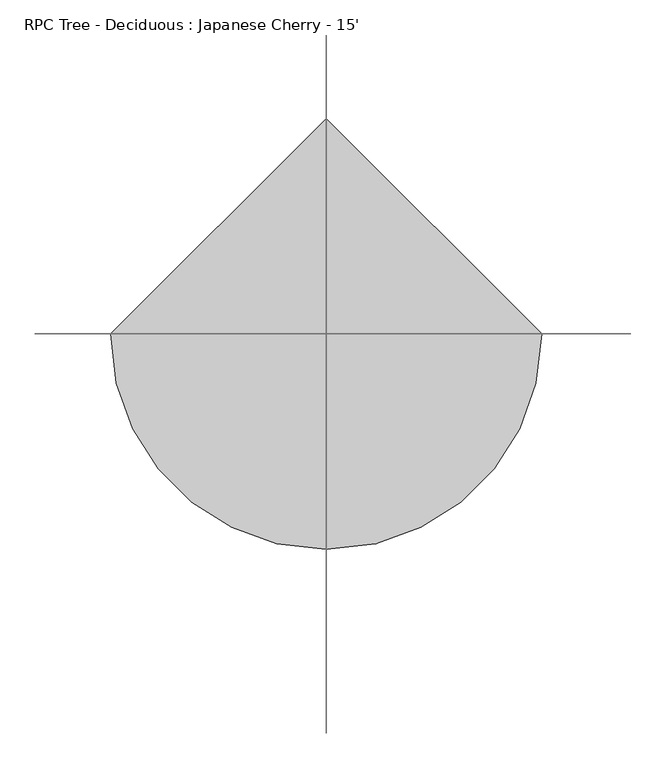
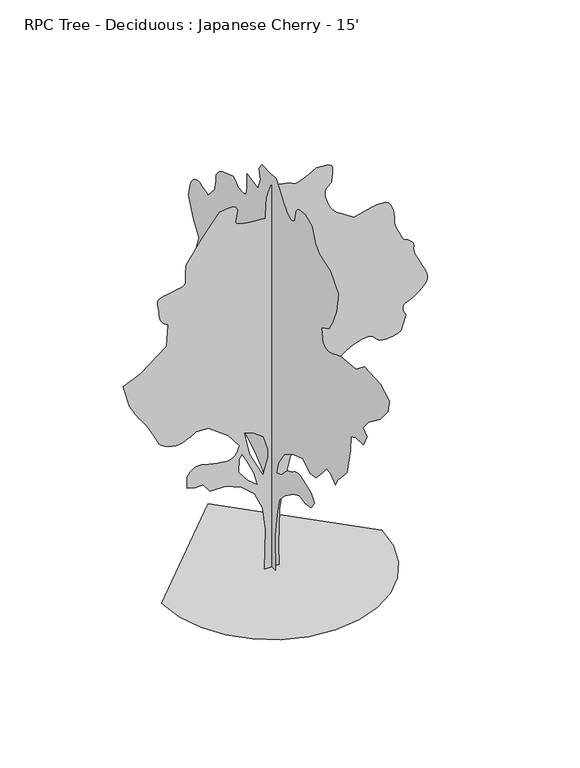
"""IFC4 building model written with IfcOpenShell, lengths in millimetres: geographic element geometry, RPC Tree - Deciduous : Japanese Cherry - 15'."""

from ifc_helpers import new_model, si_unit, origin, place, context, project, spatial, triangles, source, transform, mapped, element, save


def rpc_tree_deciduous_japanese_cherry_15_e499737d(model_context):
    return source(origin(), model_context, "Body", "Tessellation", [
        triangles([(-0.0028028, 75.7657196, 0.0059537), (-0.0028028, -73.2478183, 0.0059537), (-0.0028028, -59.7012251, 399.6312029), (-0.0028028, -100.3410047, 663.7914597), (-0.0028028, -147.7544623, 866.9916292), (-0.0028028, -256.1287339, 982.1375078), (-0.0028028, -418.6863261, 1097.2859299), (-0.0028028, -527.0605977, 1144.6976435), (-0.0028028, -635.434833, 1124.3775902), (-0.0028028, -750.5807842, 1144.6976435), (-0.0028028, -811.5407988, 1232.7519344), (-0.0028028, -750.5807842, 1314.0320023), (-0.0028028, -533.8347845, 1388.5377743), (-0.0028028, -514.9955638, 1387.0189716), (-0.0028028, -496.3341665, 1385.0834793), (-0.0028028, -478.0283798, 1382.3173691), (-0.0028028, -460.2559908, 1378.3091835), (-0.0028028, -443.1947865, 1372.6425236), (-0.0028028, -427.0200471, 1364.9005543), (-0.0028028, -411.9146828, 1354.6719635), (-0.0028028, -396.8067387, 1343.65345), (-0.0028028, -380.6345427, 1333.6991158), (-0.0028028, -363.5733384, 1324.6364422), (-0.0028028, -345.8009494, 1316.2824463), (-0.0028028, -327.4951627, 1308.4643188), (-0.0028028, -308.8337654, 1300.9992222), (-0.0028028, -289.994581, 1293.7118763), (-0.0028028, -188.3942419, 1185.3376774), (-0.0028028, -86.7944115, 1144.6976435), (-0.0028028, -127.4344454, 1286.9377258), (-0.0028028, -242.580869, 1456.2720119), (-0.0028028, -405.140496, 1557.8722057), (-0.0028028, -594.794799, 1618.8321476), (-0.0028028, -730.2607309, 1530.7779293), (-0.0028028, -838.6350025, 1544.3263756), (-0.0028028, -953.7809538, 1666.2439339), (-0.0028028, -1041.8351721, 1774.6181328), (-0.0028028, -1123.1126965, 1767.8439823), (-0.0028028, -1211.1669147, 1686.5663853), (-0.0028028, -1265.3528515, 1781.3922832), (-0.0028028, -1326.3127934, 1849.1240501), (-0.0028028, -1434.6871376, 1964.2723995), (-0.0028028, -1502.4187592, 2269.0726902), (-0.0028028, -1509.193055, 2431.6328259), (-0.0028028, -1604.0214237, 2472.2703163), (-0.0028028, -1753.0332584, 2485.8186172), (-0.0028028, -1813.9932003, 2614.5002975), (-0.0028028, -1739.4874283, 2675.4602394), (-0.0028028, -1841.0874767, 2797.3804138), (-0.0028028, -2071.3792339, 2973.5042564), (-0.0028028, -2220.3935394, 3149.6025192), (-0.0028028, -2247.4851997, 3291.8426743), (-0.0028028, -2078.1535297, 3386.6610146), (-0.0028028, -1766.5790886, 3400.2244308), (-0.0028028, -1610.7931034, 3278.3045471), (-0.0028028, -1312.7669632, 3244.4208595), (-0.0028028, -1272.2845505, 3228.5456657), (-0.0028028, -1232.7519344, 3213.2041603), (-0.0028028, -1195.1115721, 3198.9294502), (-0.0028028, -1160.3186377, 3186.2546425), (-0.0028028, -1129.3153702, 3175.7137161), (-0.0028028, -1103.0517843, 3167.8397781), (-0.0028028, -1082.4726625, 3163.1406464), (-0.0028028, -1064.0500225, 3162.8865921), (-0.0028028, -1044.5580437, 3166.9000099), (-0.0028028, -1025.4242552, 3173.6309944), (-0.0028028, -1008.065867, 3181.5558014), (-0.0028028, -993.907865, 3189.1248161), (-0.0028028, -984.3701477, 3194.789296), (-0.0028028, -980.8726141, 3197.024334), (-0.0028028, -947.0067307, 3359.5844696), (-0.0028028, -1089.2468857, 3434.0828293), (-0.0028028, -1156.9810507, 3542.4645859), (-0.0028028, -1231.4868954, 3718.5628487), (-0.0028028, -1272.127002, 3942.0832169), (-0.0028028, -1116.3410168, 4118.1814796), (-0.0028028, -913.1409199, 4192.7051285), (-0.0028028, -831.8608521, 4267.2034882), (-0.0028028, -770.9007648, 4429.7636238), (-0.0028028, -628.6606825, 4483.9417122), (-0.0028028, -605.4958537, 4483.8402649), (-0.0028028, -582.6891789, 4483.1542603), (-0.0028028, -560.5911455, 4481.2747238), (-0.0028028, -539.5599438, 4477.6426781), (-0.0028028, -519.9511116, 4471.5974075), (-0.0028028, -502.1202959, 4462.6310944), (-0.0028028, -486.4205638, 4450.0836044), (-0.0028028, -473.6824242, 4434.3863068), (-0.0028028, -464.1447433, 4416.5554184), (-0.0028028, -457.2740144, 4396.9467316), (-0.0028028, -452.5343691, 4375.9154572), (-0.0028028, -449.3949532, 4353.8173874), (-0.0028028, -447.3197528, 4331.0083145), (-0.0028028, -445.7805299, 4307.8434494), (-0.0028028, -434.0914178, 4294.9401672), (-0.0028028, -421.9248276, 4283.0531021), (-0.0028028, -408.8133096, 4273.1978897), (-0.0028028, -394.279422, 4266.3398781), (-0.0028028, -377.850701, 4263.5202827), (-0.0028028, -359.0495956, 4265.7303223), (-0.0028028, -337.4062583, 4273.9853416), (-0.0028028, -315.9610193, 4285.9741447), (-0.0028028, -297.7161846, 4298.6995308), (-0.0028028, -282.1358129, 4312.0091835), (-0.0028028, -268.6864885, 4325.8013649), (-0.0028028, -256.8373934, 4339.9237587), (-0.0028028, -246.0563473, 4354.3002068), (-0.0028028, -235.8074452, 4368.8033913), (-0.0028028, -140.9810386, 4497.5054192), (-0.0028028, -80.0209877, 4572.0037788), (-0.0028028, 21.579147, 4565.2219254), (-0.0028028, 184.1389784, 4572.0037788), (-0.0028028, 245.0987749, 4490.7235657), (-0.0028028, 218.0055885, 4375.5852448), (-0.0028028, 265.4200454, 4246.8835075), (-0.0028028, 475.3918765, 4287.5234688), (-0.0028028, 475.3918765, 4138.5014603), (-0.0028028, 476.9514107, 4115.4383331), (-0.0028028, 479.1637756, 4093.1623672), (-0.0028028, 482.6791134, 4072.5630432), (-0.0028028, 488.1502911, 4054.4781006), (-0.0028028, 496.2249435, 4039.6699928), (-0.0028028, 507.5609885, 4029.0273285), (-0.0028028, 522.8060609, 4023.3631393), (-0.0028028, 540.2228757, 4021.2551285), (-0.0028028, 557.6396542, 4020.5691238), (-0.0028028, 575.056469, 4021.0519432), (-0.0028028, 592.4732474, 4022.4995293), (-0.0028028, 609.8900259, 4024.6586998), (-0.0028028, 627.3093842, 4027.2748192), (-0.0028028, 644.726199, 4030.1449928), (-0.0028028, 660.7002239, 4045.9437378), (-0.0028028, 676.7352917, 4060.8791634), (-0.0028028, 692.8896835, 4074.0362091), (-0.0028028, 709.2193554, 4084.5265572), (-0.0028028, 725.7878208, 4091.4607269), (-0.0028028, 742.6534338, 4093.9498192), (-0.0028028, 759.8720776, 4091.1049347), (-0.0028028, 942.7522665, 4030.1449928), (-0.0028028, 968.7009007, 4012.6698967), (-0.0028028, 993.5827394, 3994.8390083), (-0.0028028, 1016.3309875, 3976.2971169), (-0.0028028, 1035.8813931, 3956.6881393), (-0.0028028, 1051.1646172, 3935.6568649), (-0.0028028, 1061.1163353, 3912.8477921), (-0.0028028, 1064.6722956, 3887.9048378), (-0.0028028, 1065.462291, 3862.3526184), (-0.0028028, 1067.6745832, 3837.8921928), (-0.0028028, 1071.0705969, 3814.3209572), (-0.0028028, 1075.4140091, 3791.4610153), (-0.0028028, 1080.4685698, 3769.1088913), (-0.0028028, 1085.9981741, 3747.1381393), (-0.0028028, 1091.7640285, 3725.3447021), (-0.0028028, 1220.4582081, 3583.1045471), (-0.0028028, 1259.5970982, 3600.2497215), (-0.0028028, 1298.4413841, 3615.8705704), (-0.0028028, 1336.691375, 3628.418351), (-0.0028028, 1374.0521759, 3636.343158), (-0.0028028, 1410.2294735, 3638.0956673), (-0.0028028, 1444.9259022, 3632.1521347), (-0.0028028, 1477.8442417, 3616.9629456), (-0.0028028, 1506.4193871, 3593.4931572), (-0.0028028, 1528.9517326, 3564.3086014), (-0.0028028, 1546.4471764, 3530.3996246), (-0.0028028, 1559.9143776, 3492.7059952), (-0.0028028, 1570.361269, 3452.1674812), (-0.0028028, 1578.7941845, 3409.7241417), (-0.0028028, 1586.218586, 3366.3410339), (-0.0028028, 1498.1643677, 3136.0643921), (-0.0028028, 1389.7926395, 2987.0423836), (-0.0028028, 1477.8442417, 2743.2023254), (-0.0028028, 1396.5641739, 2614.5002975), (-0.0028028, 1363.3893093, 2602.8164177), (-0.0028028, 1331.4588455, 2590.6497185), (-0.0028028, 1302.0151485, 2577.543251), (-0.0028028, 1276.3027645, 2563.0144867), (-0.0028028, 1255.5687103, 2546.5806061), (-0.0028028, 1241.0552067, 2527.7820442), (-0.0028028, 1234.0040382, 2506.1385979), (-0.0028028, 1231.6953129, 2483.1135498), (-0.0028028, 1230.4506214, 2460.4416779), (-0.0028028, 1230.0949745, 2438.0692062), (-0.0028028, 1230.4506214, 2415.9330574), (-0.0028028, 1231.339666, 2393.9721886), (-0.0028028, 1232.5842121, 2372.13326), (-0.0028028, 1234.0040382, 2350.3502872), (-0.0028028, 1206.9124506, 2241.9785591), (-0.0028028, 1017.2581112, 2262.2985397), (-0.0028028, 1001.4999161, 2230.5052769), (-0.0028028, 986.9863398, 2199.5401611), (-0.0028028, 974.9594576, 2170.2361359), (-0.0028028, 966.6663591, 2143.4188774), (-0.0028028, 963.3491198, 2119.9211838), (-0.0028028, 966.2523582, 2100.5664059), (-0.0028028, 976.6180773, 2086.1925739), (-0.0028028, 993.4227201, 2074.2646683), (-0.0028028, 1014.0196461, 2062.1005852), (-0.0028028, 1037.2225176, 2050.292149), (-0.0028028, 1061.8478313, 2039.431184), (-0.0028028, 1086.7093952, 2030.1093693), (-0.0028028, 1110.6234879, 2022.9211452), (-0.0028028, 1132.4039898, 2018.4583363), (-0.0028028, 1152.1322187, 2014.567004), (-0.0028028, 1170.7936523, 2008.9003441), (-0.0028028, 1188.5660414, 2001.7526699), (-0.0028028, 1205.6272093, 1993.4190216), (-0.0028028, 1222.157523, 1984.1961834), (-0.0028028, 1238.3297916, 1974.3816662), (-0.0028028, 1254.3241642, 1964.2723995), (-0.0028028, 1410.1126202, 2045.5524673), (-0.0028028, 1454.8979679, 2056.9850544), (-0.0028028, 1498.4412403, 2067.3533169), (-0.0028028, 1539.4952751, 2075.5879887), (-0.0028028, 1576.817997, 2080.6222744), (-0.0028028, 1609.1650051, 2081.3919949), (-0.0028028, 1635.2914627, 2076.8326801), (-0.0028028, 1653.9502075, 2065.8725933), (-0.0028028, 1666.2946575, 2049.9747265), (-0.0028028, 1674.7249569, 2031.5900928), (-0.0028028, 1679.8989143, 2011.1329113), (-0.0028028, 1682.4669262, 1989.0146393), (-0.0028028, 1683.0789528, 1965.6542919), (-0.0028028, 1682.3881519, 1941.4631813), (-0.0028028, 1681.0444839, 1916.8582878), (-0.0028028, 1657.7627655, 1892.3904499), (-0.0028028, 1634.1255455, 1869.1697742), (-0.0028028, 1609.7770317, 1848.4331039), (-0.0028028, 1584.3618679, 1831.4303627), (-0.0028028, 1557.5241165, 1819.4059513), (-0.0028028, 1528.9110374, 1813.5996197), (-0.0028028, 1498.1643677, 1815.2582394), (-0.0028028, 1465.6015297, 1822.4057682), (-0.0028028, 1432.5637207, 1830.9782101), (-0.0028028, 1400.2370602, 1839.0732101), (-0.0028028, 1369.8078129, 1844.8009129), (-0.0028028, 1342.4571568, 1846.2614342), (-0.0028028, 1319.3735367, 1841.5624477), (-0.0028028, 1301.7382759, 1828.8040695), (-0.0028028, 1288.4084209, 1812.3752758), (-0.0028028, 1277.2120113, 1797.7219551), (-0.0028028, 1267.7912201, 1784.5521194), (-0.0028028, 1259.7953419, 1772.5657871), (-0.0028028, 1252.8636429, 1761.4660286), (-0.0028028, 1246.6430923, 1750.9605652), (-0.0028028, 1240.778334, 1740.752322), (-0.0028028, 1263.8618088, 1737.6916077), (-0.0028028, 1286.1172817, 1733.6834221), (-0.0028028, 1306.714135, 1727.7779686), (-0.0028028, 1324.821896, 1719.0302467), (-0.0028028, 1339.6122723, 1706.4901691), (-0.0028028, 1350.2574074, 1689.2105553), (-0.0028028, 1355.9242126, 1666.2439339), (-0.0028028, 1358.2355541, 1639.3300243), (-0.0028028, 1359.4802456, 1610.9912018), (-0.0028028, 1359.8357471, 1581.4687305), (-0.0028028, 1359.4802456, 1550.9989334), (-0.0028028, 1358.591201, 1519.8178425), (-0.0028028, 1357.3466549, 1488.1643967), (-0.0028028, 1355.9242126, 1456.2720119), (-0.0028028, 1321.1312782, 1430.3436527), (-0.0028028, 1286.5720505, 1405.5990875), (-0.0028028, 1252.4876484, 1383.2266159), (-0.0028028, 1219.1146128, 1364.4078518), (-0.0028028, 1186.6915192, 1350.328624), (-0.0028028, 1155.4494581, 1342.1725811), (-0.0028028, 1125.6323828, 1341.1261333), (-0.0028028, 1095.812764, 1344.8167511), (-0.0028028, 1064.5732464, 1349.9322819), (-0.0028028, 1032.1476093, 1356.2316067), (-0.0028028, 998.774501, 1363.478112), (-0.0028028, 964.6902443, 1371.4385273), (-0.0028028, 930.1334873, 1379.8688267), (-0.0028028, 895.3380095, 1388.5377743), (-0.0028028, 692.1378399, 1341.1261333), (-0.0028028, 455.0718596, 1219.2061043), (-0.0028028, 319.6059277, 1144.6976435), (-0.0028028, 163.8189614, 1016.005862), (-0.0028028, 68.9922959, 819.5799156), (-0.0028028, 41.8991095, 541.8713216), (-0.0028028, 68.9922959, 264.1652892), (80.2102203, 0.0002552, 0.0), (-82.349661, 0.0002552, 0.0), (-68.8030678, 0.0002233, 460.5862032), (-102.6694236, 0.000202, 724.7463873), (-190.7229152, 0.0001914, 914.3981833), (-332.9637969, 0.0001914, 1043.0925081), (-509.0697627, 0.0001807, 1117.5983528), (-678.4015417, 0.0001807, 1117.5983528), (-759.684153, 0.0001807, 1219.1984013), (-847.7358278, 0.0001807, 1219.1984013), (-935.7901188, 0.0001807, 1239.5183819), (-935.7901188, 0.0001701, 1368.2127068), (-918.2539072, 0.0001701, 1391.2175526), (-900.0065472, 0.0001701, 1412.9192802), (-880.3392883, 0.0001595, 1432.0150623), (-858.5384388, 0.0001595, 1447.2017807), (-833.8928501, 0.0001595, 1457.1737011), (-805.6936993, 0.0001595, 1460.6307575), (-773.2299831, 0.0001595, 1456.266925), (-734.6829174, 0.0001595, 1446.5108345), (-690.4487715, 0.0001595, 1435.4516258), (-643.1335636, 0.0001701, 1424.2757092), (-595.3460009, 0.0001701, 1414.1639717), (-549.689449, 0.0001701, 1406.3051491), (-508.7725788, 0.0001701, 1401.8804192), (-475.2013721, 0.0001701, 1402.0785175), (-448.544024, 0.0001701, 1408.1415195), (-426.1513865, 0.0001701, 1419.8916744), (-407.3122021, 0.0001595, 1436.3813656), (-391.3152497, 0.0001595, 1456.660651), (-377.4544679, 0.0001595, 1479.7848209), (-365.0135485, 0.0001595, 1504.8039333), (-353.2838139, 0.0001595, 1530.7728424), (-475.2013721, 0.0001488, 1693.3329781), (-698.7215223, 0.0001382, 1855.8931137), (-834.1899977, 0.0001382, 1862.6647934), (-856.0492739, 0.0001382, 1849.6320133), (-878.4419477, 0.0001382, 1836.7771294), (-901.9038877, 0.0001382, 1824.277747), (-926.9610065, 0.0001382, 1812.3092915), (-954.1543322, 0.0001382, 1801.0544552), (-984.01203, 0.0001382, 1790.6861927), (-1017.0701866, 0.0001488, 1781.3847256), (-1055.1015862, 0.0001488, 1778.1664627), (-1097.4002398, 0.0001488, 1784.6638859), (-1140.7656887, 0.0001382, 1798.9792912), (-1182.0000904, 0.0001382, 1819.2206429), (-1217.9005154, 0.0001382, 1843.490237), (-1245.2690483, 0.0001382, 1869.8935673), (-1260.907774, 0.0001382, 1896.5332203), (-1274.5551968, 0.0001382, 1929.7461639), (-1296.2570698, 0.0001276, 1973.9803825), (-1323.2903034, 0.0001276, 2024.4959038), (-1352.9320988, 0.0001276, 2076.5482498), (-1382.45457, 0.0001276, 2125.4025352), (-1409.1321568, 0.0001169, 2166.3195145), (-1430.2420601, 0.0001169, 2194.5592152), (-1448.055217, 0.0001169, 2217.0508656), (-1466.5769062, 0.0001169, 2243.4541958), (-1485.6928905, 0.0001169, 2273.113868), (-1505.2813751, 0.0001169, 2305.3794857), (-1525.2255066, 0.0001063, 2339.6035595), (-1545.4082863, 0.0001063, 2375.12799), (-1565.7080647, 0.0001063, 2411.3051422), (-1640.2164528, 9.57e-05, 2668.7039658), (-1443.7878902, 8.51e-05, 2749.9838882), (-1159.310269, 7.44e-05, 2973.5042564), (-1145.7618954, 5.32e-05, 3217.3190254), (-1165.9447477, 5.32e-05, 3231.9748169), (-1185.2970549, 5.32e-05, 3247.3163223), (-1202.9906696, 5.32e-05, 3264.0804153), (-1218.1951195, 5.32e-05, 3282.9780991), (-1230.0823299, 5.32e-05, 3304.7203766), (-1237.8242992, 5.32e-05, 3330.0188324), (-1240.5902641, 5.32e-05, 3359.5591805), (-1243.0389519, 4.25e-05, 3392.8330215), (-1248.5659401, 4.25e-05, 3427.5294502), (-1254.4511913, 4.25e-05, 3461.7686394), (-1257.9665291, 4.25e-05, 3493.6204742), (-1256.3865383, 4.25e-05, 3521.204837), (-1246.9860947, 4.25e-05, 3542.6169022), (-1227.0419632, 4.25e-05, 3556.002713), (-1192.1092844, 4.25e-05, 3564.4103394), (-1144.1438982, 3.19e-05, 3572.715937), (-1090.0164608, 3.19e-05, 3581.5808029), (-1036.6002445, 3.19e-05, 3591.7915169), (-990.7659056, 3.19e-05, 3603.9835052), (-959.3867163, 3.19e-05, 3618.9186401), (-949.3359489, 3.19e-05, 3637.2829262), (-951.449192, 3.19e-05, 3659.3809959), (-952.1400656, 3.19e-05, 3684.6794518), (-951.644747, 3.19e-05, 3712.6448959), (-950.2045732, 3.19e-05, 3742.718351), (-948.0532511, 2.13e-05, 3774.4175789), (-945.4268852, 2.13e-05, 3807.1836021), (-942.5617258, 2.13e-05, 3840.4830231), (-773.2299831, 1.06e-05, 4084.3233719), (-576.803964, -1.06e-05, 4328.16343), (-534.9980856, -1.06e-05, 4335.1231796), (-494.9117606, -1.06e-05, 4340.3809982), (-458.2595647, -1.06e-05, 4342.2096657), (-426.7635221, -1.06e-05, 4338.8569633), (-402.1382083, -1.06e-05, 4328.6459587), (-386.1031769, -1.06e-05, 4309.850013), (-380.3754742, 0.0, 4280.7416153), (-383.1999384, 0.0, 4247.9503029), (-389.6972889, 0.0, 4219.0450905), (-396.9057878, 0.0, 4193.848082), (-401.8613357, 0.0, 4172.0549355), (-401.6048106, 0.0, 4153.462175), (-393.1720041, 0.0, 4137.8410355), (-373.6038308, 0.0, 4124.9633331), (-343.9238837, 0.0, 4114.5238541), (-307.8431645, 0.0, 4106.2435455), (-266.4335192, 1.06e-05, 4099.7157463), (-220.7586908, 1.06e-05, 4094.6355331), (-171.883967, 1.06e-05, 4090.5971169), (-120.8766607, 1.06e-05, 4087.2697037), (-68.8030678, 1.06e-05, 4084.3233719), (-62.0293897, 0.0, 4267.2034882), (-60.4495079, -1.06e-05, 4293.1367889), (-56.0260951, -1.06e-05, 4318.689299), (-49.2331141, -1.06e-05, 4343.962175), (-40.544273, -1.06e-05, 4369.0065765), (-30.4335416, -1.06e-05, 4393.8733727), (-19.3751868, -1.06e-05, 4418.612851), (-7.8427643, -1.06e-05, 4443.3017509), (38.3857792, -1.06e-05, 4434.5642029), (83.3110485, -1.06e-05, 4425.7249168), (125.6295138, -1.06e-05, 4416.6571564), (164.0381523, -1.06e-05, 4407.2083145), (197.2334371, -1.06e-05, 4397.3022331), (223.9120957, -1.06e-05, 4386.7865959), (242.7705922, -1.06e-05, 4375.5599556), (267.3174405, -1.06e-05, 4372.2834114), (307.2640574, -1.06e-05, 4382.5194145), (355.6256767, -1.06e-05, 4401.5188362), (405.4097383, -1.06e-05, 4424.5566742), (449.6235366, -1.06e-05, 4446.8576385), (481.2770551, -2.13e-05, 4463.7234695), (493.3827115, -2.13e-05, 4470.4035851), (503.1388384, -2.13e-05, 4470.6067703), (528.2975498, -2.13e-05, 4470.3274269), (562.6967946, -2.13e-05, 4468.2699944), (600.177065, -2.13e-05, 4463.1392029), (634.5763098, -1.06e-05, 4453.6142029), (659.7350212, -1.06e-05, 4438.3994339), (669.4911844, -1.06e-05, 4416.1999168), (669.0949877, -1.06e-05, 4390.4698013), (667.9900406, -1.06e-05, 4365.4506889), (666.2907984, -1.06e-05, 4341.0411324), (664.1190559, -1.06e-05, 4317.089106), (661.5918119, -1.06e-05, 4293.4922905), (658.8257017, 0.0, 4270.1245308), (655.9428108, 0.0, 4246.8835075), (638.6835445, 0.0, 4233.6753021), (622.3741476, 0.0, 4219.7308044), (607.9571134, 0.0, 4204.2114029), (596.3848546, 0.0, 4186.4060944), (588.6048426, 0.0, 4165.5271362), (585.5644395, 0.0, 4140.7876579), (588.2111166, 0.0, 4111.3996262), (595.5949319, 1.06e-05, 4078.8367882), (605.8235227, 1.06e-05, 4045.6643944), (618.4244614, 1.06e-05, 4012.9492401), (632.9176901, 1.06e-05, 3981.7834099), (648.8333611, 1.06e-05, 3953.233699), (665.698974, 1.06e-05, 3928.3416138), (683.0370146, 2.13e-05, 3908.1995293), (703.4154945, 2.13e-05, 3889.8099541), (729.1278786, 2.13e-05, 3869.6170006), (759.2802532, 2.13e-05, 3847.9505905), (792.9912043, 2.13e-05, 3825.1159378), (829.3639841, 2.13e-05, 3801.3670967), (867.5148531, 2.13e-05, 3777.0592781), (906.5572374, 2.13e-05, 3752.4212471), (974.48703, 2.13e-05, 3771.0140076), (1040.6997763, 2.13e-05, 3787.8795479), (1103.475959, 2.13e-05, 3801.2909386), (1161.1010027, 2.13e-05, 3809.5712471), (1211.8502306, 2.13e-05, 3810.9682549), (1254.0116833, 2.13e-05, 3803.7800308), (1285.8633728, 2.13e-05, 3786.2793549), (1308.8096466, 2.13e-05, 3757.831382), (1325.9495888, 3.19e-05, 3721.2045479), (1338.1136719, 3.19e-05, 3679.8280037), (1346.1325138, 3.19e-05, 3637.155899), (1350.8315002, 3.19e-05, 3596.6173851), (1353.0438652, 4.25e-05, 3561.641613), (1353.5976105, 4.25e-05, 3535.6827324), (1358.8503422, 4.25e-05, 3507.9969223), (1372.3961723, 4.25e-05, 3469.2870758), (1390.9178616, 4.25e-05, 3425.1418053), (1411.1006413, 5.32e-05, 3381.0982727), (1429.6249466, 5.32e-05, 3342.7442184), (1443.1707767, 5.32e-05, 3315.6423843), (1448.4235085, 5.32e-05, 3305.3808014), (1455.5126106, 5.32e-05, 3302.5614967), (1473.6202263, 5.32e-05, 3294.4079247), (1498.0094353, 5.32e-05, 3281.4031952), (1523.9376492, 5.32e-05, 3264.0042572), (1546.6656223, 5.32e-05, 3242.6936394), (1561.456144, 5.32e-05, 3217.9538704), (1563.5693871, 6.38e-05, 3190.2424805), (1560.9227463, 6.38e-05, 3161.8962456), (1563.9655838, 6.38e-05, 3134.3880409), (1571.7456322, 6.38e-05, 3106.8795456), (1583.3178909, 6.38e-05, 3078.5585999), (1597.7324181, 6.38e-05, 3048.5613029), (1614.0443584, 7.44e-05, 3016.0746231), (1631.3036247, 7.44e-05, 2980.2605301), (1651.0114334, 7.44e-05, 2941.4239471), (1672.8529781, 7.44e-05, 2900.911013), (1693.1526112, 7.44e-05, 2859.5850471), (1708.2377369, 8.51e-05, 2818.2593719), (1714.4404106, 8.51e-05, 2777.7461472), (1708.0801884, 8.51e-05, 2738.9095642), (1685.4894161, 8.51e-05, 2702.5620735), (1655.0603142, 9.57e-05, 2670.8884254), (1626.9983643, 9.57e-05, 2644.9042557), (1600.3587112, 9.57e-05, 2623.6442162), (1574.1941746, 9.57e-05, 2606.1944092), (1547.5546669, 9.57e-05, 2591.5894867), (1519.4951878, 9.57e-05, 2578.8641006), (1489.0634697, 9.57e-05, 2567.103772), (1463.2545799, 9.57e-05, 2553.5147758), (1448.4615875, 9.57e-05, 2536.3646599), (1442.8532089, 9.57e-05, 2516.2632706), (1444.5930737, 0.0001063, 2493.7893517), (1451.8397243, 0.0001063, 2469.5399597), (1462.7592613, 0.0001063, 2444.1069191), (1475.5176395, 0.0001063, 2418.079438), (1421.329232, 0.0001169, 2248.7450066), (1402.2741451, 0.0001169, 2240.1167542), (1382.0913654, 0.0001169, 2231.9607113), (1359.6579964, 0.0001169, 2224.752285), (1333.8491066, 0.0001169, 2218.9661556), (1303.5367126, 0.0001169, 2215.0772942), (1267.5955925, 0.0001169, 2213.5558754), (1224.9032856, 0.0001169, 2214.8791958), (1186.5543182, 0.0001169, 2223.6651421), (1160.2907324, 0.0001169, 2241.2216286), (1139.9504042, 0.0001169, 2263.0426804), (1119.3738258, 0.0001169, 2284.6250839), (1092.3990189, 0.0001169, 2301.470422), (1052.8638594, 0.0001169, 2309.0727196), (994.6089123, 0.0001169, 2302.9309433), (927.2531399, 0.0001169, 2283.7970821), (865.4625074, 0.0001169, 2256.8426228), (810.6645441, 0.0001169, 2224.1985397), (764.2764599, 0.0001169, 2188.0035107), (727.7258566, 0.0001169, 2150.3835686), (702.4274008, 0.0001276, 2113.4772457), (689.8112377, 0.0001276, 2079.4133366), (689.5343651, 0.0001276, 2049.0602474), (699.2092106, 0.0001276, 2021.5520428), (717.179698, 0.0001276, 1996.4136063), (741.7847368, 0.0001276, 1973.172583), (771.3655621, 0.0001382, 1951.3515312), (804.2662428, 0.0001382, 1930.4778053), (838.8229998, 0.0001382, 1910.0790504), (858.9855045, 0.0001382, 1896.9268009), (878.2006107, 0.0001382, 1883.2412991), (895.5183764, 0.0001382, 1868.4914726), (909.9938009, 0.0001382, 1852.1415985), (920.6770878, 0.0001382, 1833.6579884), (926.620693, 0.0001382, 1812.5073898), (926.8772181, 0.0001382, 1788.158876), (924.1721506, 0.0001488, 1758.4790016), (921.8225847, 0.0001488, 1722.4008259), (919.7677683, 0.0001488, 1680.9911442), (917.9516727, 0.0001488, 1635.3142811), (916.3107845, 0.0001595, 1586.4395027), (914.7919092, 0.0001595, 1535.4337498), (913.3288445, 0.0001595, 1483.3585854), (878.4571358, 0.0001595, 1457.529348), (843.3467062, 0.0001595, 1433.4780544), (807.7613056, 0.0001701, 1412.980323), (771.4646839, 0.0001701, 1397.8139523), (734.2231344, 0.0001701, 1389.7570312), (695.792922, 0.0001701, 1390.585033), (655.9428108, 0.0001701, 1402.0785175), (615.8971447, 0.0001701, 1417.3236626), (576.9157305, 0.0001701, 1428.6597439), (538.820781, 0.0001595, 1436.7368671), (501.4395962, 0.0001595, 1442.205574), (464.5917727, 0.0001595, 1445.7209118), (428.0995597, 0.0001595, 1447.9332767), (391.7826267, 0.0001595, 1449.4927746), (276.6366936, 0.0001701, 1374.9868572), (202.1305764, 0.0001807, 1205.6525711), (127.6236689, 0.0001914, 921.1724064), (86.9838894, 0.0002126, 643.4663195), (73.4370464, 0.0002339, 237.0665254), (-95.8962542, 8.51e-05, 1097.2783722), (-41.7096271, 7.44e-05, 1286.9326389), (-41.7096271, 6.38e-05, 1381.7585369), (-89.122576, 5.32e-05, 1544.3186726), (-211.0424234, 5.32e-05, 1632.3728909), (-305.8695931, 5.32e-05, 1666.238847), (-244.9095423, 6.38e-05, 1395.3069832), (-156.8557963, 6.38e-05, 1009.2266247), (-197.4958302, 6.38e-05, 1158.2383867), (-272.003746, 5.32e-05, 1320.7984497), (-326.1896101, 4.25e-05, 1422.3986435), (-360.0554572, 4.25e-05, 1374.9868572), (-366.829644, 5.32e-05, 1225.9725517), (-265.2295592, 6.38e-05, 1097.2783722), (-1212.9170259, 0.0, 0.0045929), (-1180.85205, -277.9194097, 0.0045929), (-1089.5287725, -533.1464181, 0.0045929), (-946.2625174, -758.3633034, 0.0045929), (-758.3633034, -946.2625174, 0.0045929), (-533.1464181, -1089.5287725, 0.0045929), (-277.9194097, -1180.85205, 0.0045929), (5.3e-05, -1212.9170259, 0.0045929), (277.9194097, -1180.85205, 0.0045929), (533.1464181, -1089.5287725, 0.0045929), (758.3633034, -946.2625174, 0.0045929), (946.2625174, -758.3633034, 0.0045929), (1089.5287725, -533.1464181, 0.0045929), (1180.85205, -277.9194097, 0.0045929), (1212.9170259, 0.0001063, 0.0045929), (-0.0001591, 1212.9170259, 0.0045929)], [[38, 39, 40], [115, 116, 117], [1, 2, 3], [280, 1, 3], [279, 280, 3], [279, 3, 4], [278, 279, 4], [278, 4, 5], [186, 187, 188], [277, 278, 5], [46, 47, 48], [45, 46, 48], [277, 5, 6], [185, 186, 188], [10, 11, 12], [9, 10, 12], [9, 12, 13], [8, 9, 13], [8, 13, 14], [8, 14, 15], [8, 15, 16], [8, 16, 17], [8, 17, 18], [8, 18, 19], [8, 19, 20], [8, 20, 21], [7, 8, 21], [7, 21, 22], [7, 22, 23], [7, 23, 24], [7, 24, 25], [7, 25, 26], [6, 7, 26], [6, 26, 27], [6, 27, 28], [277, 6, 28], [277, 28, 29], [51, 52, 53], [50, 51, 53], [50, 53, 54], [50, 54, 55], [49, 50, 55], [49, 55, 56], [48, 49, 56], [48, 56, 57], [45, 48, 57], [44, 45, 57], [44, 57, 58], [44, 58, 59], [44, 59, 60], [44, 60, 61], [44, 61, 62], [44, 62, 63], [276, 277, 29], [276, 29, 30], [184, 185, 188], [183, 184, 188], [44, 63, 64], [115, 117, 118], [111, 112, 113], [111, 113, 114], [182, 183, 188], [109, 110, 111], [109, 111, 114], [108, 109, 114], [108, 114, 115], [107, 108, 115], [106, 107, 115], [105, 106, 115], [104, 105, 115], [115, 118, 119], [170, 171, 172], [170, 172, 173], [170, 173, 174], [170, 174, 175], [74, 75, 76], [74, 76, 77], [73, 74, 77], [72, 73, 77], [71, 72, 77], [258, 259, 260], [181, 182, 188], [78, 79, 80], [170, 175, 176], [103, 104, 115], [78, 80, 81], [44, 64, 65], [275, 276, 30], [275, 30, 31], [274, 275, 31], [78, 81, 82], [78, 82, 83], [78, 83, 84], [78, 84, 85], [78, 85, 86], [78, 86, 87], [78, 87, 88], [78, 88, 89], [78, 89, 90], [78, 90, 91], [78, 91, 92], [78, 92, 93], [78, 93, 94], [78, 94, 95], [78, 95, 96], [71, 77, 78], [71, 78, 96], [71, 96, 97], [71, 97, 98], [71, 98, 99], [71, 99, 100], [115, 119, 120], [180, 181, 188], [38, 40, 41], [223, 224, 225], [33, 34, 35], [33, 35, 36], [33, 36, 37], [102, 103, 115], [179, 180, 188], [44, 65, 66], [170, 176, 177], [71, 100, 101], [43, 44, 66], [42, 43, 66], [41, 42, 66], [38, 41, 66], [37, 38, 66], [33, 37, 66], [33, 66, 67], [33, 67, 68], [33, 68, 69], [33, 69, 70], [32, 33, 70], [31, 32, 70], [274, 31, 70], [273, 274, 70], [273, 70, 71], [273, 71, 101], [273, 101, 102], [273, 102, 115], [273, 115, 120], [273, 120, 121], [273, 121, 122], [273, 122, 123], [273, 123, 124], [273, 124, 125], [273, 125, 126], [273, 126, 127], [273, 127, 128], [273, 128, 129], [273, 129, 130], [273, 130, 131], [272, 273, 131], [271, 272, 131], [270, 271, 131], [269, 270, 131], [268, 269, 131], [268, 131, 132], [268, 132, 133], [268, 133, 134], [167, 168, 169], [257, 258, 260], [257, 260, 261], [256, 257, 261], [256, 261, 262], [255, 256, 262], [255, 262, 263], [254, 255, 263], [254, 263, 264], [254, 264, 265], [254, 265, 266], [254, 266, 267], [254, 267, 268], [253, 254, 268], [252, 253, 268], [251, 252, 268], [250, 251, 268], [249, 250, 268], [248, 249, 268], [247, 248, 268], [246, 247, 268], [245, 246, 268], [166, 167, 169], [165, 166, 169], [164, 165, 169], [163, 164, 169], [162, 163, 169], [161, 162, 169], [160, 161, 169], [159, 160, 169], [158, 159, 169], [157, 158, 169], [156, 157, 169], [155, 156, 169], [154, 155, 169], [154, 169, 170], [154, 170, 177], [153, 154, 177], [153, 177, 178], [153, 178, 179], [153, 179, 188], [222, 223, 225], [222, 225, 226], [221, 222, 226], [220, 221, 226], [219, 220, 226], [218, 219, 226], [217, 218, 226], [216, 217, 226], [215, 216, 226], [214, 215, 226], [213, 214, 226], [212, 213, 226], [212, 226, 227], [212, 227, 228], [212, 228, 229], [212, 229, 230], [212, 230, 231], [211, 212, 231], [211, 231, 232], [211, 232, 233], [210, 211, 233], [209, 210, 233], [209, 233, 234], [209, 234, 235], [209, 235, 236], [209, 236, 237], [209, 237, 238], [209, 238, 239], [209, 239, 240], [208, 209, 240], [208, 240, 241], [207, 208, 241], [206, 207, 241], [206, 241, 242], [205, 206, 242], [204, 205, 242], [204, 242, 243], [203, 204, 243], [202, 203, 243], [202, 243, 244], [201, 202, 244], [201, 244, 245], [201, 245, 268], [200, 201, 268], [199, 200, 268], [198, 199, 268], [197, 198, 268], [196, 197, 268], [195, 196, 268], [194, 195, 268], [153, 188, 189], [153, 189, 190], [152, 153, 190], [152, 190, 191], [151, 152, 191], [136, 137, 138], [135, 136, 138], [135, 138, 139], [134, 135, 139], [134, 139, 140], [134, 140, 141], [134, 141, 142], [134, 142, 143], [134, 143, 144], [134, 144, 145], [134, 145, 146], [134, 146, 147], [134, 147, 148], [134, 148, 149], [134, 149, 150], [134, 150, 151], [134, 151, 191], [134, 191, 192], [134, 192, 193], [268, 134, 193], [194, 268, 193], [583, 580, 581], [574, 281, 575], [580, 583, 584], [573, 574, 575], [583, 581, 575], [580, 584, 585], [572, 573, 575], [582, 583, 575], [582, 575, 281], [571, 572, 575], [571, 575, 576], [281, 282, 283], [570, 571, 576], [570, 576, 577], [344, 345, 346], [290, 291, 292], [406, 407, 408], [570, 577, 578], [290, 292, 293], [289, 290, 293], [289, 293, 294], [289, 294, 295], [289, 295, 296], [289, 296, 297], [289, 297, 298], [289, 298, 299], [289, 299, 300], [289, 300, 301], [289, 301, 302], [289, 302, 303], [288, 289, 303], [287, 288, 303], [287, 303, 304], [287, 304, 305], [287, 305, 306], [286, 287, 306], [286, 306, 307], [286, 307, 308], [286, 308, 309], [569, 570, 578], [554, 555, 556], [405, 406, 408], [343, 344, 346], [512, 513, 514], [511, 512, 514], [511, 514, 515], [511, 515, 516], [511, 516, 517], [510, 511, 517], [510, 517, 518], [510, 518, 519], [510, 519, 520], [510, 520, 521], [510, 521, 522], [510, 522, 523], [510, 523, 524], [509, 510, 524], [509, 524, 525], [508, 509, 525], [434, 435, 436], [342, 343, 346], [507, 508, 525], [507, 525, 526], [405, 408, 409], [404, 405, 409], [403, 404, 409], [403, 409, 410], [402, 403, 410], [401, 402, 410], [400, 401, 410], [400, 410, 411], [399, 400, 411], [399, 411, 412], [399, 412, 413], [399, 413, 414], [399, 414, 415], [377, 378, 379], [341, 342, 346], [341, 346, 347], [340, 341, 347], [339, 340, 347], [338, 339, 347], [337, 338, 347], [336, 337, 347], [335, 336, 347], [334, 335, 347], [333, 334, 347], [377, 379, 380], [377, 380, 381], [377, 381, 382], [377, 382, 383], [377, 383, 384], [377, 384, 385], [377, 385, 386], [377, 386, 387], [377, 387, 388], [377, 388, 389], [377, 389, 390], [377, 390, 391], [376, 377, 391], [376, 391, 392], [375, 376, 392], [374, 375, 392], [373, 374, 392], [372, 373, 392], [372, 392, 393], [371, 372, 393], [370, 371, 393], [369, 370, 393], [369, 393, 394], [369, 394, 395], [369, 395, 396], [332, 333, 347], [369, 396, 397], [426, 427, 428], [426, 428, 429], [425, 426, 429], [425, 429, 430], [424, 425, 430], [424, 430, 431], [423, 424, 431], [423, 431, 432], [422, 423, 432], [422, 432, 433], [421, 422, 433], [420, 421, 433], [419, 420, 433], [418, 419, 433], [418, 433, 434], [418, 434, 436], [418, 436, 437], [418, 437, 438], [418, 438, 439], [417, 418, 439], [417, 439, 440], [416, 417, 440], [416, 440, 441], [415, 416, 441], [399, 415, 441], [399, 441, 442], [399, 442, 443], [399, 443, 444], [399, 444, 445], [399, 445, 446], [399, 446, 447], [399, 447, 448], [399, 448, 449], [369, 397, 398], [331, 332, 347], [368, 369, 398], [360, 361, 362], [359, 360, 362], [359, 362, 363], [358, 359, 363], [358, 363, 364], [357, 358, 364], [357, 364, 365], [356, 357, 365], [355, 356, 365], [355, 365, 366], [354, 355, 366], [353, 354, 366], [352, 353, 366], [351, 352, 366], [350, 351, 366], [349, 350, 366], [348, 349, 366], [348, 366, 367], [348, 367, 368], [348, 368, 398], [347, 348, 398], [347, 398, 399], [347, 399, 449], [347, 449, 450], [347, 450, 451], [347, 451, 452], [331, 347, 452], [331, 452, 453], [331, 453, 454], [331, 454, 455], [331, 455, 456], [330, 331, 456], [329, 330, 456], [328, 329, 456], [327, 328, 456], [326, 327, 456], [325, 326, 456], [324, 325, 456], [323, 324, 456], [322, 323, 456], [321, 322, 456], [320, 321, 456], [319, 320, 456], [318, 319, 456], [317, 318, 456], [316, 317, 456], [315, 316, 456], [314, 315, 456], [314, 456, 457], [314, 457, 458], [314, 458, 459], [314, 459, 460], [314, 460, 461], [314, 461, 462], [314, 462, 463], [314, 463, 464], [314, 464, 465], [314, 465, 466], [314, 466, 467], [314, 467, 468], [314, 468, 469], [314, 469, 470], [314, 470, 471], [314, 471, 472], [314, 472, 473], [314, 473, 474], [314, 474, 475], [314, 475, 476], [314, 476, 477], [314, 477, 478], [314, 478, 479], [314, 479, 480], [314, 480, 481], [314, 481, 482], [314, 482, 483], [314, 483, 484], [314, 484, 485], [314, 485, 486], [314, 486, 487], [314, 487, 488], [314, 488, 489], [314, 489, 490], [314, 490, 491], [314, 491, 492], [314, 492, 493], [314, 493, 494], [314, 494, 495], [314, 495, 496], [314, 496, 497], [314, 497, 498], [314, 498, 499], [314, 499, 500], [314, 500, 501], [314, 501, 502], [580, 585, 586], [554, 556, 557], [553, 554, 557], [553, 557, 558], [553, 558, 559], [553, 559, 560], [553, 560, 561], [553, 561, 562], [553, 562, 563], [552, 553, 563], [552, 563, 564], [551, 552, 564], [550, 551, 564], [550, 564, 565], [549, 550, 565], [549, 565, 566], [548, 549, 566], [547, 548, 566], [546, 547, 566], [545, 546, 566], [544, 545, 566], [543, 544, 566], [542, 543, 566], [541, 542, 566], [540, 541, 566], [539, 540, 566], [538, 539, 566], [538, 566, 567], [537, 538, 567], [537, 567, 568], [537, 568, 569], [537, 569, 578], [536, 537, 578], [535, 536, 578], [535, 578, 579], [534, 535, 579], [534, 579, 580], [533, 534, 580], [532, 533, 580], [507, 526, 527], [506, 507, 527], [531, 532, 580], [506, 527, 528], [530, 531, 580], [281, 283, 284], [582, 281, 284], [582, 284, 285], [582, 285, 286], [588, 582, 286], [587, 588, 286], [587, 286, 309], [586, 587, 309], [586, 309, 310], [586, 310, 311], [586, 311, 312], [586, 312, 313], [580, 586, 313], [580, 313, 314], [530, 580, 314], [529, 530, 314], [502, 503, 504], [502, 504, 505], [314, 502, 505], [529, 314, 505], [529, 505, 506], [529, 506, 528], [603, 604, 589], [602, 603, 589], [602, 589, 590], [601, 602, 590], [601, 590, 591], [601, 591, 592], [600, 601, 592], [599, 600, 592], [599, 592, 593], [599, 593, 594], [599, 594, 595], [599, 595, 596], [599, 596, 597], [599, 597, 598]], closed=False),
    ])


if __name__ == "__main__":
    model = new_model("IFC4")
    model_context = context("Model", 3, world=origin())
    ifc_project = project(units=[si_unit("LENGTHUNIT", "METRE", prefix="MILLI")], contexts=[model_context])
    site = spatial("IfcSite", under=ifc_project)
    building = spatial("IfcBuilding", under=site)
    placement = place(None, origin())
    rpc_tree_deciduous_japanese_cherry_15_shape = rpc_tree_deciduous_japanese_cherry_15_e499737d(model_context)
    element("IfcGeographicElement", 1, ObjectType="RPC Tree - Deciduous : Japanese Cherry - 15'", at=placement, inside=building, context=model_context, shape_type="MappedRepresentation", body=[
        mapped(rpc_tree_deciduous_japanese_cherry_15_shape, transform((0.0, 0.0, 0.0), x_axis=(1.0, 0.0, 0.0), y_axis=(0.0, 1.0, 0.0), z_axis=(0.0, 0.0, 1.0))),
    ])
    save(model, "model.ifc")

# Revit data of these elements
# Type "RPC Tree - Deciduous : Japanese Cherry - 15'"
#   built-in parameter 1005198 = "{2, 15},{39, RPC-16-FXGW-2MQ0-PN7K-A000-ST1L-LVER-AU},{1, 0},{1, 0},{2, 35},{1, 8},{5, Color},{1, 0},{1, 0},{3, 0.8},{3, 0.8},{3, 0.8},{1, 8},{7, BBoxMin},{1, 0},{1, 0},{1, 0},{1, 0},{1, 0},{1, 8},{7, BBoxMax},{1, 0},{1, 0},{1, 0},{1, 0},{1, 0},{2, 11},{9, RPCTypeId},{1, 0},{1, 0},{39, RPC-16-FXGW-2MQ0-PN7K-A000-ST1L-LVER-AU},{1, 6},{14, RPCPlantHeight},{1, 0},{1, 0},{2, 15},{2, 11},{7, keyword},{1, 0},{1, 0},{207, :Geometry:RPC:Japanese Flowering Cherry:Prunus serrulata Lindl:A landscape tree:valued for its abundant showy flowers; native to China and Japan.  Hardy only in the mildest parts of Canada and farther south.},{2, 11},{8, category},{1, 0},{1, 0},{16, :Trees [General]},{2, 11},{12, LocalizedUID},{1, 0},{1, 0},{25, Japanese Flowering Cherry},{2, 14},{6, Height},{1, 0},{1, 0},{2, 15},{1, 2},{16, Cast Reflections},{1, 0},{1, 0},{1, 0},{1, 2},{12, Cast Shadows},{1, 0},{1, 0},{1, 1},{1, 2},{9, Lock View},{1, 0},{1, 0},{1, 0},{1, 4},{5, ViewC},{1, 0},{1, 0},{1, 0},{2, 11},{20, AdvancedUIDefinition},{1, 0},{1, 0},{0, },{2, 11},{10, AssetLibID},{1, 0},{1, 0},{36, 4D3F6E72-3F99-4203-98E9-AF80B3C7A7A4},{2, 11},{10, BaseSchema},{1, 0},{1, 0},{9, RPCSchema},{2, 11},{12, ExchangeGUID},{1, 0},{1, 0},{0, },{1, 2},{6, Hidden},{1, 0},{1, 0},{1, 0},{1, 4},{11, RPCCategory},{1, 0},{1, 0},{1, 0},{2, 11},{8, RPCImage},{1, 0},{1, 0},{0, },{1, 4},{13, SchemaVersion},{1, 0},{1, 0},{1, 4},{2, 11},{12, UIDefinition},{1, 0},{1, 0},{0, },{2, 11},{6, UIName},{1, 0},{1, 0},{39, RPC-16-FXGW-2MQ0-PN7K-A000-ST1L-LVER-AU},{2, 11},{11, VersionGUID},{1, 0},{1, 0},{9, RPCSchema},{2, 11},{9, assettype},{1, 0},{1, 0},{11, RPCGeometry},{2, 11},{11, description},{1, 0},{1, 0},{0, },{2, 11},{9, localname},{1, 0},{1, 0},{3, RPC},{2, 11},{9, localtype},{1, 0},{1, 0},{3, RPC},{1, 4},{8, revision},{1, 0},{1, 0},{1, 1},{2, 11},{9, thumbnail},{1, 0},{1, 0},{0, },{1, 4},{7, version},{1, 0},{1, 0},{1, 1},{1, 2},{20, RPC_Cast Reflections},{1, 0},{1, 0},{1, 1},{1, 2},{16, RPC_Cast Shadows},{1, 0},{1, 0},{1, 1},{1, 2},{13, RPC_Lock View},{1, 0},{1, 0},{1, 0},{1, 4},{9, RPC_ViewC},{1, 0},{1, 0},{1, 0},{21, assetlibrary_base.fbx},{1, 5},"
#   built-in parameter 1005195 = "RPC-16-FXGW-2MQ0-PN7K-A000-ST1L-LVER-AU"
#   Type Comments = "Japanese Cherry"
#   Assembly Code = "G2050500"
#   Height = 15' - 0"
#   Default Elevation = 0
